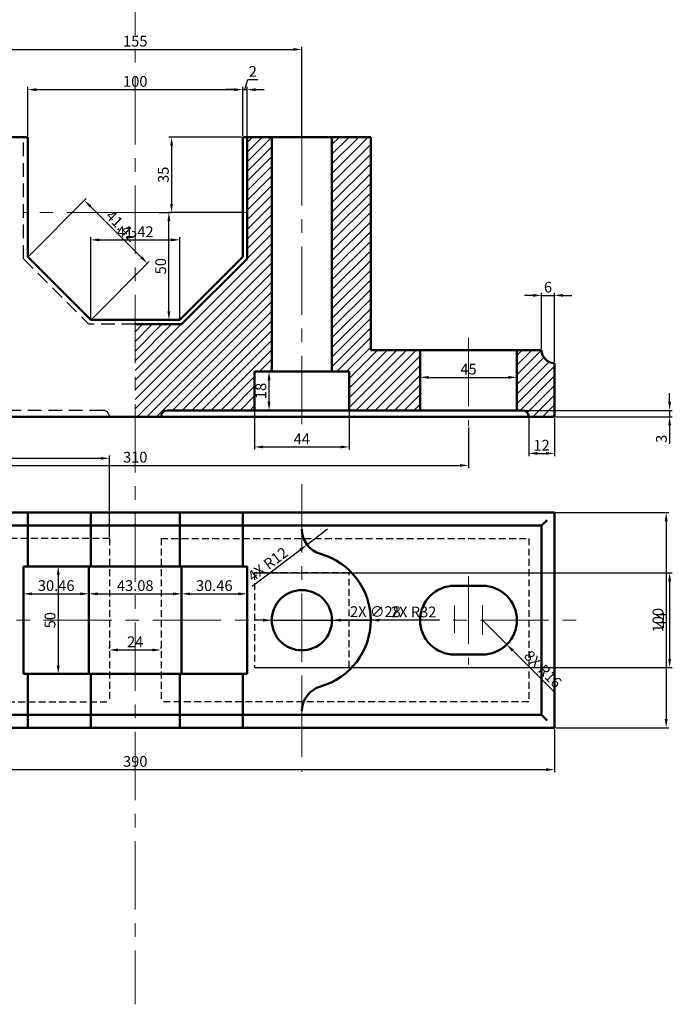
# Model space of a CAD drawing. Units: millimetres. Extents: x 3191 to 3694, y 1533 to 2269.
# Tile 2 of 2: x 3390 to 3694, y 1533 to 1990. Entities that reach past the tile are written whole.
import ezdxf

# ---------------------------------------------------------------- set-up
doc = ezdxf.new("R2010")
doc.units = ezdxf.units.MM
doc.linetypes.add('CENTER', pattern=[50.8, 31.75, -6.35, 6.35, -6.35])
doc.linetypes.add('HIDDEN', pattern=[9.525, 6.35, -3.175])
for name, color, linetype, lineweight in [('M-CNTR', 4, 'CENTER', 18), ('M-DIMS', 2, 'Continuous', 25), ('M-HATC', 8, 'Continuous', 18), ('M-HIDN', 3, 'HIDDEN', 25), ('M-OUTL', 7, 'Continuous', 50)]:
    doc.layers.add(name, color=color, linetype=linetype, lineweight=lineweight)
doc.styles.get("Standard").update_dxf_attribs({"font": 'arial.ttf'})
doc.dimstyles.new('ISO-25', dxfattribs={"dimtxt": 5, "dimasz": 4, "dimexe": 1.25, "dimexo": 0.625, "dimtad": 1, "dimdsep": 46, "dimtxsty": 'Standard', "dimcen": 2.5, "dimadec": 0, "dimazin": 0, "dimtfac": 1, "dimtmove": 0, "dimatfit": 3, "dimfxl": 1, "dimarcsym": 0})

# ---------------------------------------------------------------- blocks, each defined once
blk = doc.blocks.new('*D1')
at = {"layer": 'Defpoints', "color": 0, "ltscale": 0.5, "transparency": 16777216}
for p in [(3431.85, 1697.44), (3455.85, 1697.44), (3455.85, 1697.44)]:
    blk.add_point(p, dxfattribs=at)
at = {"layer": 'M-DIMS', "color": 0, "lineweight": -2, "ltscale": 0.5, "transparency": 16777216}
for p, q in [((3431.85, 1698.07), (3431.85, 1698.69)), ((3455.85, 1698.07), (3455.85, 1698.69)), ((3435.85, 1697.44), (3451.85, 1697.44))]:
    blk.add_line(p, q, dxfattribs=at)
at = {"layer": 'M-DIMS', "color": 0, "ltscale": 0.5, "transparency": 16777216}
for points in [[(3435.85, 1698.11), (3435.85, 1696.77), (3431.85, 1697.44)], [(3451.85, 1698.11), (3451.85, 1696.77), (3455.85, 1697.44)]]:
    blk.add_solid(points, dxfattribs=at)
at = {"layer": 'M-DIMS', "color": 0, "ltscale": 0.5, "transparency": 16777216, "insert": (3443.85, 1700.58), "char_height": 5, "attachment_point": 5}
blk.add_mtext('24', dxfattribs=at)
blk = doc.blocks.new('*D2')
at = {"layer": 'Defpoints', "color": 0, "ltscale": 0.5, "transparency": 16777216}
for p in [(3288.85, 1800.04), (3598.85, 1801.48), (3598.85, 1783.23)]:
    blk.add_point(p, dxfattribs=at)
at = {"layer": 'M-DIMS', "color": 0, "lineweight": -2, "ltscale": 0.5, "transparency": 16777216}
for p, q in [((3288.85, 1799.41), (3288.85, 1781.98)), ((3598.85, 1800.86), (3598.85, 1781.98)), ((3292.85, 1783.23), (3594.85, 1783.23))]:
    blk.add_line(p, q, dxfattribs=at)
at = {"layer": 'M-DIMS', "color": 0, "ltscale": 0.5, "transparency": 16777216}
for points in [[(3292.85, 1783.9), (3292.85, 1782.57), (3288.85, 1783.23)], [(3594.85, 1783.9), (3594.85, 1782.57), (3598.85, 1783.23)]]:
    blk.add_solid(points, dxfattribs=at)
at = {"layer": 'M-DIMS', "color": 0, "ltscale": 0.5, "transparency": 16777216, "insert": (3443.85, 1786.41), "char_height": 5, "attachment_point": 5}
blk.add_mtext('310', dxfattribs=at)
blk = doc.blocks.new('*D6')
at = {"layer": 'Defpoints', "color": 0, "ltscale": 0.5, "transparency": 16777216}
for p in [(3521.35, 1976.6), (3366.35, 1935.82), (3521.35, 1935.82)]:
    blk.add_point(p, dxfattribs=at)
at = {"layer": 'M-DIMS', "color": 0, "lineweight": -2, "ltscale": 0.5, "transparency": 16777216}
for p, q in [((3366.35, 1936.45), (3366.35, 1977.85)), ((3521.35, 1936.45), (3521.35, 1977.85)), ((3370.35, 1976.6), (3517.35, 1976.6))]:
    blk.add_line(p, q, dxfattribs=at)
at = {"layer": 'M-DIMS', "color": 0, "ltscale": 0.5, "transparency": 16777216}
for points in [[(3370.35, 1977.27), (3370.35, 1975.93), (3366.35, 1976.6)], [(3517.35, 1977.27), (3517.35, 1975.93), (3521.35, 1976.6)]]:
    blk.add_solid(points, dxfattribs=at)
at = {"layer": 'M-DIMS', "color": 0, "ltscale": 0.5, "transparency": 16777216, "insert": (3443.85, 1979.78), "char_height": 5, "attachment_point": 5}
blk.add_mtext('155', dxfattribs=at)
blk = doc.blocks.new('*D7')
at = {"layer": 'Defpoints', "color": 0, "ltscale": 0.5, "transparency": 16777216}
for p in [(3493.85, 1957.9), (3393.85, 1935.81), (3493.85, 1935.81)]:
    blk.add_point(p, dxfattribs=at)
at = {"layer": 'M-DIMS', "color": 0, "lineweight": -2, "ltscale": 0.5, "transparency": 16777216}
for p, q in [((3393.85, 1936.43), (3393.85, 1959.15)), ((3493.85, 1936.43), (3493.85, 1959.15)), ((3397.85, 1957.9), (3489.85, 1957.9))]:
    blk.add_line(p, q, dxfattribs=at)
at = {"layer": 'M-DIMS', "color": 0, "ltscale": 0.5, "transparency": 16777216}
for points in [[(3397.85, 1958.56), (3397.85, 1957.23), (3393.85, 1957.9)], [(3489.85, 1958.56), (3489.85, 1957.23), (3493.85, 1957.9)]]:
    blk.add_solid(points, dxfattribs=at)
at = {"layer": 'M-DIMS', "color": 0, "ltscale": 0.5, "transparency": 16777216, "insert": (3443.85, 1961.08), "char_height": 5, "attachment_point": 5}
blk.add_mtext('100', dxfattribs=at)
blk = doc.blocks.new('*D8')
at = {"layer": 'Defpoints', "color": 0, "ltscale": 0.5, "transparency": 16777216}
for p in [(3495.85, 1957.9), (3493.85, 1935.81), (3495.85, 1935.82)]:
    blk.add_point(p, dxfattribs=at)
at = {"layer": 'M-DIMS', "color": 0, "lineweight": -2, "ltscale": 0.5, "transparency": 16777216}
for p, q in [((3493.85, 1936.43), (3493.85, 1959.15)), ((3494.85, 1957.9), (3496.26, 1962.6)), ((3495.85, 1936.45), (3495.85, 1959.15)), ((3496.26, 1962.6), (3500.83, 1962.6)), ((3489.85, 1957.9), (3485.85, 1957.9)), ((3493.85, 1957.9), (3495.85, 1957.9)), ((3493.85, 1957.9), (3495.85, 1957.9)), ((3499.85, 1957.9), (3503.85, 1957.9))]:
    blk.add_line(p, q, dxfattribs=at)
at = {"layer": 'M-DIMS', "color": 0, "ltscale": 0.5, "transparency": 16777216}
for points in [[(3489.85, 1958.56), (3489.85, 1957.23), (3493.85, 1957.9)], [(3499.85, 1958.56), (3499.85, 1957.23), (3495.85, 1957.9)]]:
    blk.add_solid(points, dxfattribs=at)
at = {"layer": 'M-DIMS', "color": 0, "ltscale": 0.5, "transparency": 16777216, "insert": (3498.54, 1965.73), "char_height": 5, "attachment_point": 5}
blk.add_mtext('2', dxfattribs=at)
blk = doc.blocks.new('*D9')
at = {"layer": 'Defpoints', "color": 0, "ltscale": 0.5, "transparency": 16777216}
for p in [(3454.21, 1900.82), (3459.5, 1900.82), (3454.21, 1850.82)]:
    blk.add_point(p, dxfattribs=at)
at = {"layer": 'M-DIMS', "color": 0, "lineweight": -2, "ltscale": 0.5, "transparency": 16777216}
for p, q in [((3454.83, 1900.82), (3460.75, 1900.82)), ((3459.5, 1854.82), (3459.5, 1896.82)), ((3454.83, 1850.82), (3460.75, 1850.82))]:
    blk.add_line(p, q, dxfattribs=at)
at = {"layer": 'M-DIMS', "color": 0, "ltscale": 0.5, "transparency": 16777216}
for points in [[(3458.84, 1896.82), (3460.17, 1896.82), (3459.5, 1900.82)], [(3458.84, 1854.82), (3460.17, 1854.82), (3459.5, 1850.82)]]:
    blk.add_solid(points, dxfattribs=at)
at = {"layer": 'M-DIMS', "color": 0, "ltscale": 0.5, "transparency": 16777216, "insert": (3456.33, 1875.82), "char_height": 5, "attachment_point": 5, "rotation": 90}
blk.add_mtext('50', dxfattribs=at)
blk = doc.blocks.new('*D10')
at = {"layer": 'Defpoints', "color": 0, "ltscale": 0.5, "transparency": 16777216}
for p in [(3493.85, 1935.82), (3460.75, 1900.82), (3493.85, 1900.82)]:
    blk.add_point(p, dxfattribs=at)
at = {"layer": 'M-DIMS', "color": 0, "lineweight": -2, "ltscale": 0.5, "transparency": 16777216}
for p, q in [((3493.23, 1935.82), (3459.5, 1935.82)), ((3460.75, 1931.82), (3460.75, 1904.82)), ((3493.23, 1900.82), (3459.5, 1900.82))]:
    blk.add_line(p, q, dxfattribs=at)
at = {"layer": 'M-DIMS', "color": 0, "ltscale": 0.5, "transparency": 16777216}
for points in [[(3460.09, 1931.82), (3461.42, 1931.82), (3460.75, 1935.82)], [(3460.09, 1904.82), (3461.42, 1904.82), (3460.75, 1900.82)]]:
    blk.add_solid(points, dxfattribs=at)
at = {"layer": 'M-DIMS', "color": 0, "ltscale": 0.5, "transparency": 16777216, "insert": (3457.57, 1918.32), "char_height": 5, "attachment_point": 5, "rotation": 90}
blk.add_mtext('35', dxfattribs=at)
blk = doc.blocks.new('*D11')
at = {"layer": 'Defpoints', "color": 0, "ltscale": 0.5, "transparency": 16777216}
for p in [(3576.35, 1822.82), (3621.35, 1824.16), (3621.35, 1822.82)]:
    blk.add_point(p, dxfattribs=at)
at = {"layer": 'M-DIMS', "color": 0, "lineweight": -2, "ltscale": 0.5, "transparency": 16777216}
for p, q in [((3576.35, 1823.45), (3576.35, 1825.41)), ((3580.35, 1824.16), (3617.35, 1824.16)), ((3621.35, 1823.45), (3621.35, 1825.41))]:
    blk.add_line(p, q, dxfattribs=at)
at = {"layer": 'M-DIMS', "color": 0, "ltscale": 0.5, "transparency": 16777216}
for points in [[(3580.35, 1824.82), (3580.35, 1823.49), (3576.35, 1824.16)], [(3617.35, 1824.82), (3617.35, 1823.49), (3621.35, 1824.16)]]:
    blk.add_solid(points, dxfattribs=at)
at = {"layer": 'M-DIMS', "color": 0, "ltscale": 0.5, "transparency": 16777216, "insert": (3598.85, 1827.32), "char_height": 5, "attachment_point": 5}
blk.add_mtext('45', dxfattribs=at)
blk = doc.blocks.new('*D12')
at = {"layer": 'Defpoints', "color": 0, "ltscale": 0.5, "transparency": 16777216}
for p in [(3626.85, 1805.82), (3638.85, 1805.82), (3638.85, 1788.81)]:
    blk.add_point(p, dxfattribs=at)
at = {"layer": 'M-DIMS', "color": 0, "lineweight": -2, "ltscale": 0.5, "transparency": 16777216}
for p, q in [((3626.85, 1805.2), (3626.85, 1787.56)), ((3638.85, 1805.2), (3638.85, 1787.56)), ((3630.85, 1788.81), (3634.85, 1788.81))]:
    blk.add_line(p, q, dxfattribs=at)
at = {"layer": 'M-DIMS', "color": 0, "ltscale": 0.5, "transparency": 16777216}
for points in [[(3630.85, 1789.48), (3630.85, 1788.15), (3626.85, 1788.81)], [(3634.85, 1789.48), (3634.85, 1788.15), (3638.85, 1788.81)]]:
    blk.add_solid(points, dxfattribs=at)
at = {"layer": 'M-DIMS', "color": 0, "ltscale": 0.5, "transparency": 16777216, "insert": (3632.85, 1791.95), "char_height": 5, "attachment_point": 5}
blk.add_mtext('12', dxfattribs=at)
blk = doc.blocks.new('*D13')
at = {"layer": 'Defpoints', "color": 0, "ltscale": 0.5, "transparency": 16777216}
for p in [(3638.85, 1862.26), (3632.85, 1836.82), (3638.85, 1830.82)]:
    blk.add_point(p, dxfattribs=at)
at = {"layer": 'M-DIMS', "color": 0, "lineweight": -2, "ltscale": 0.5, "transparency": 16777216}
for p, q in [((3632.85, 1837.45), (3632.85, 1863.51)), ((3638.85, 1831.45), (3638.85, 1863.51)), ((3628.85, 1862.26), (3624.85, 1862.26)), ((3632.85, 1862.26), (3638.85, 1862.26)), ((3642.85, 1862.26), (3646.85, 1862.26))]:
    blk.add_line(p, q, dxfattribs=at)
at = {"layer": 'M-DIMS', "color": 0, "ltscale": 0.5, "transparency": 16777216}
for points in [[(3628.85, 1862.93), (3628.85, 1861.59), (3632.85, 1862.26)], [(3642.85, 1862.93), (3642.85, 1861.59), (3638.85, 1862.26)]]:
    blk.add_solid(points, dxfattribs=at)
at = {"layer": 'M-DIMS', "color": 0, "ltscale": 0.5, "transparency": 16777216, "insert": (3635.85, 1865.44), "char_height": 5, "attachment_point": 5}
blk.add_mtext('6', dxfattribs=at)
blk = doc.blocks.new('*D14')
at = {"layer": 'Defpoints', "color": 0, "ltscale": 0.5, "transparency": 16777216}
for p in [(3499.35, 1808.82), (3543.35, 1808.82), (3543.35, 1791.8)]:
    blk.add_point(p, dxfattribs=at)
at = {"layer": 'M-DIMS', "color": 0, "lineweight": -2, "ltscale": 0.5, "transparency": 16777216}
for p, q in [((3499.35, 1808.2), (3499.35, 1790.55)), ((3543.35, 1808.2), (3543.35, 1790.55)), ((3503.35, 1791.8), (3539.35, 1791.8))]:
    blk.add_line(p, q, dxfattribs=at)
at = {"layer": 'M-DIMS', "color": 0, "ltscale": 0.5, "transparency": 16777216}
for points in [[(3503.35, 1792.47), (3503.35, 1791.13), (3499.35, 1791.8)], [(3539.35, 1792.47), (3539.35, 1791.13), (3543.35, 1791.8)]]:
    blk.add_solid(points, dxfattribs=at)
at = {"layer": 'M-DIMS', "color": 0, "ltscale": 0.5, "transparency": 16777216, "insert": (3521.35, 1794.93), "char_height": 5, "attachment_point": 5}
blk.add_mtext('44', dxfattribs=at)
blk = doc.blocks.new('*D15')
at = {"layer": 'Defpoints', "color": 0, "ltscale": 0.5, "transparency": 16777216}
for p in [(3638.85, 1761.27), (3638.85, 1661.27), (3690.8, 1661.27)]:
    blk.add_point(p, dxfattribs=at)
at = {"layer": 'M-DIMS', "color": 0, "lineweight": -2, "ltscale": 0.5, "transparency": 16777216}
for p, q in [((3639.48, 1761.27), (3692.05, 1761.27)), ((3690.8, 1757.27), (3690.8, 1665.27)), ((3639.48, 1661.27), (3692.05, 1661.27))]:
    blk.add_line(p, q, dxfattribs=at)
at = {"layer": 'M-DIMS', "color": 0, "ltscale": 0.5, "transparency": 16777216}
for points in [[(3690.13, 1757.27), (3691.46, 1757.27), (3690.8, 1761.27)], [(3690.13, 1665.27), (3691.46, 1665.27), (3690.8, 1661.27)]]:
    blk.add_solid(points, dxfattribs=at)
at = {"layer": 'M-DIMS', "color": 0, "ltscale": 0.5, "transparency": 16777216, "insert": (3687.62, 1711.27), "char_height": 5, "attachment_point": 5, "rotation": 90}
blk.add_mtext('100', dxfattribs=at)
blk = doc.blocks.new('*D16')
at = {"layer": 'Defpoints', "color": 0, "ltscale": 0.5, "transparency": 16777216}
for p in [(3408.03, 1736.27), (3408.03, 1686.27), (3408.03, 1686.27)]:
    blk.add_point(p, dxfattribs=at)
at = {"layer": 'M-DIMS', "color": 0, "lineweight": -2, "ltscale": 0.5, "transparency": 16777216}
for p, q in [((3408.66, 1736.27), (3409.28, 1736.27)), ((3408.03, 1732.27), (3408.03, 1690.27)), ((3408.66, 1686.27), (3409.28, 1686.27))]:
    blk.add_line(p, q, dxfattribs=at)
at = {"layer": 'M-DIMS', "color": 0, "ltscale": 0.5, "transparency": 16777216}
for points in [[(3407.37, 1732.27), (3408.7, 1732.27), (3408.03, 1736.27)], [(3407.37, 1690.27), (3408.7, 1690.27), (3408.03, 1686.27)]]:
    blk.add_solid(points, dxfattribs=at)
at = {"layer": 'M-DIMS', "color": 0, "ltscale": 0.5, "transparency": 16777216, "insert": (3404.86, 1711.27), "char_height": 5, "attachment_point": 5, "rotation": 90}
blk.add_mtext('50', dxfattribs=at)
blk = doc.blocks.new('*D20')
at = {"layer": 'Defpoints', "color": 0, "ltscale": 0.5, "transparency": 16777216}
for p in [(3248.85, 1661.27), (3638.85, 1661.27), (3638.85, 1641.8)]:
    blk.add_point(p, dxfattribs=at)
at = {"layer": 'M-DIMS', "color": 0, "lineweight": -2, "ltscale": 0.5, "transparency": 16777216}
for p, q in [((3248.85, 1660.65), (3248.85, 1640.55)), ((3638.85, 1660.65), (3638.85, 1640.55)), ((3252.85, 1641.8), (3634.85, 1641.8))]:
    blk.add_line(p, q, dxfattribs=at)
at = {"layer": 'M-DIMS', "color": 0, "ltscale": 0.5, "transparency": 16777216}
for points in [[(3252.85, 1642.47), (3252.85, 1641.14), (3248.85, 1641.8)], [(3634.85, 1642.47), (3634.85, 1641.14), (3638.85, 1641.8)]]:
    blk.add_solid(points, dxfattribs=at)
at = {"layer": 'M-DIMS', "color": 0, "ltscale": 0.5, "transparency": 16777216, "insert": (3443.85, 1644.98), "char_height": 5, "attachment_point": 5}
blk.add_mtext('390', dxfattribs=at)
blk = doc.blocks.new('*D22')
at = {"layer": 'Defpoints', "color": 0, "ltscale": 0.5, "transparency": 16777216}
for p in [(3464.56, 1888.07), (3423.14, 1850.82), (3464.56, 1850.82)]:
    blk.add_point(p, dxfattribs=at)
at = {"layer": 'M-DIMS', "color": 0, "lineweight": -2, "ltscale": 0.5, "transparency": 16777216}
for p, q in [((3423.14, 1851.45), (3423.14, 1889.32)), ((3427.14, 1888.07), (3460.56, 1888.07)), ((3464.56, 1851.45), (3464.56, 1889.32))]:
    blk.add_line(p, q, dxfattribs=at)
at = {"layer": 'M-DIMS', "color": 0, "ltscale": 0.5, "transparency": 16777216}
for points in [[(3427.14, 1888.74), (3427.14, 1887.4), (3423.14, 1888.07)], [(3460.56, 1888.74), (3460.56, 1887.4), (3464.56, 1888.07)]]:
    blk.add_solid(points, dxfattribs=at)
at = {"layer": 'M-DIMS', "color": 0, "ltscale": 0.5, "transparency": 16777216, "insert": (3443.85, 1891.21), "char_height": 5, "attachment_point": 5}
blk.add_mtext('41.42', dxfattribs=at)
blk = doc.blocks.new('*D23')
at = {"layer": 'Defpoints', "color": 0, "ltscale": 0.5, "transparency": 16777216}
for p in [(3393.85, 1880.11), (3449.48, 1877.16), (3423.14, 1850.82)]:
    blk.add_point(p, dxfattribs=at)
at = {"layer": 'M-DIMS', "color": 0, "lineweight": -2, "ltscale": 0.5, "transparency": 16777216}
for p, q in [((3394.3, 1880.55), (3421.08, 1907.33)), ((3423.02, 1903.62), (3446.65, 1879.99)), ((3423.59, 1851.26), (3450.37, 1878.04))]:
    blk.add_line(p, q, dxfattribs=at)
at = {"layer": 'M-DIMS', "color": 0, "ltscale": 0.5, "transparency": 16777216}
for points in [[(3423.49, 1904.09), (3422.55, 1903.15), (3420.19, 1906.45)], [(3447.13, 1880.46), (3446.18, 1879.52), (3449.48, 1877.16)]]:
    blk.add_solid(points, dxfattribs=at)
at = {"layer": 'M-DIMS', "color": 0, "ltscale": 0.5, "transparency": 16777216, "insert": (3437.06, 1894.02), "char_height": 5, "attachment_point": 5, "rotation": 315}
blk.add_mtext('41.42', dxfattribs=at)
blk = doc.blocks.new('*D24')
at = {"layer": 'Defpoints', "color": 0, "ltscale": 0.5, "transparency": 16777216}
for p in [(3506.1, 1826.82), (3543.35, 1826.82), (3543.35, 1808.82)]:
    blk.add_point(p, dxfattribs=at)
at = {"layer": 'M-DIMS', "color": 0, "lineweight": -2, "ltscale": 0.5, "transparency": 16777216}
for p, q in [((3542.73, 1826.82), (3504.85, 1826.82)), ((3506.1, 1812.82), (3506.1, 1822.82)), ((3542.73, 1808.82), (3504.85, 1808.82))]:
    blk.add_line(p, q, dxfattribs=at)
at = {"layer": 'M-DIMS', "color": 0, "ltscale": 0.5, "transparency": 16777216}
for points in [[(3505.44, 1822.82), (3506.77, 1822.82), (3506.1, 1826.82)], [(3505.44, 1812.82), (3506.77, 1812.82), (3506.1, 1808.82)]]:
    blk.add_solid(points, dxfattribs=at)
at = {"layer": 'M-DIMS', "color": 0, "ltscale": 0.5, "transparency": 16777216, "insert": (3502.93, 1817.82), "char_height": 5, "attachment_point": 5, "rotation": 90}
blk.add_mtext('18', dxfattribs=at)
blk = doc.blocks.new('*D25')
at = {"layer": 'Defpoints', "color": 0, "ltscale": 0.5, "transparency": 16777216}
for p in [(3623.85, 1808.82), (3638.85, 1805.82), (3692.41, 1805.82)]:
    blk.add_point(p, dxfattribs=at)
at = {"layer": 'M-DIMS', "color": 0, "lineweight": -2, "ltscale": 0.5, "transparency": 16777216}
for p, q in [((3692.41, 1812.82), (3692.41, 1816.82)), ((3624.48, 1808.82), (3693.66, 1808.82)), ((3692.41, 1808.82), (3692.41, 1805.82)), ((3639.48, 1805.82), (3693.66, 1805.82)), ((3692.41, 1801.82), (3692.41, 1793.3))]:
    blk.add_line(p, q, dxfattribs=at)
at = {"layer": 'M-DIMS', "color": 0, "ltscale": 0.5, "transparency": 16777216}
for points in [[(3691.74, 1812.82), (3693.07, 1812.82), (3692.41, 1808.82)], [(3691.74, 1801.82), (3693.07, 1801.82), (3692.41, 1805.82)]]:
    blk.add_solid(points, dxfattribs=at)
at = {"layer": 'M-DIMS', "color": 0, "ltscale": 0.5, "transparency": 16777216, "insert": (3689.23, 1795.56), "char_height": 5, "attachment_point": 5, "rotation": 90}
blk.add_mtext('3', dxfattribs=at)
blk = doc.blocks.new('*D26')
at = {"layer": 'Defpoints', "color": 0, "ltscale": 0.5, "transparency": 16777216}
for p in [(3422.32, 1723.52), (3391.85, 1686.27), (3422.32, 1686.27)]:
    blk.add_point(p, dxfattribs=at)
at = {"layer": 'M-DIMS', "color": 0, "lineweight": -2, "ltscale": 0.5, "transparency": 16777216}
for p, q in [((3391.85, 1686.9), (3391.85, 1724.77)), ((3395.85, 1723.52), (3418.32, 1723.52)), ((3422.32, 1686.9), (3422.32, 1724.77))]:
    blk.add_line(p, q, dxfattribs=at)
at = {"layer": 'M-DIMS', "color": 0, "ltscale": 0.5, "transparency": 16777216}
for points in [[(3395.85, 1724.19), (3395.85, 1722.86), (3391.85, 1723.52)], [(3418.32, 1724.19), (3418.32, 1722.86), (3422.32, 1723.52)]]:
    blk.add_solid(points, dxfattribs=at)
at = {"layer": 'M-DIMS', "color": 0, "ltscale": 0.5, "transparency": 16777216, "insert": (3407.08, 1726.7), "char_height": 5, "attachment_point": 5}
blk.add_mtext('30.46', dxfattribs=at)
blk = doc.blocks.new('*D27')
at = {"layer": 'Defpoints', "color": 0, "ltscale": 0.5, "transparency": 16777216}
for p in [(3465.39, 1723.52), (3422.32, 1686.27), (3465.39, 1686.27)]:
    blk.add_point(p, dxfattribs=at)
at = {"layer": 'M-DIMS', "color": 0, "lineweight": -2, "ltscale": 0.5, "transparency": 16777216}
for p, q in [((3422.32, 1686.9), (3422.32, 1724.77)), ((3426.32, 1723.52), (3461.39, 1723.52)), ((3465.39, 1686.9), (3465.39, 1724.77))]:
    blk.add_line(p, q, dxfattribs=at)
at = {"layer": 'M-DIMS', "color": 0, "ltscale": 0.5, "transparency": 16777216}
for points in [[(3426.32, 1724.19), (3426.32, 1722.86), (3422.32, 1723.52)], [(3461.39, 1724.19), (3461.39, 1722.86), (3465.39, 1723.52)]]:
    blk.add_solid(points, dxfattribs=at)
at = {"layer": 'M-DIMS', "color": 0, "ltscale": 0.5, "transparency": 16777216, "insert": (3443.85, 1726.7), "char_height": 5, "attachment_point": 5}
blk.add_mtext('43.08', dxfattribs=at)
blk = doc.blocks.new('*D28')
at = {"layer": 'Defpoints', "color": 0, "ltscale": 0.5, "transparency": 16777216}
for p in [(3495.85, 1723.52), (3465.39, 1686.27), (3495.85, 1686.27)]:
    blk.add_point(p, dxfattribs=at)
at = {"layer": 'M-DIMS', "color": 0, "lineweight": -2, "ltscale": 0.5, "transparency": 16777216}
for p, q in [((3465.39, 1686.9), (3465.39, 1724.77)), ((3469.39, 1723.52), (3491.85, 1723.52)), ((3495.85, 1686.9), (3495.85, 1724.77))]:
    blk.add_line(p, q, dxfattribs=at)
at = {"layer": 'M-DIMS', "color": 0, "ltscale": 0.5, "transparency": 16777216}
for points in [[(3469.39, 1724.19), (3469.39, 1722.86), (3465.39, 1723.52)], [(3491.85, 1724.19), (3491.85, 1722.86), (3495.85, 1723.52)]]:
    blk.add_solid(points, dxfattribs=at)
at = {"layer": 'M-DIMS', "color": 0, "ltscale": 0.5, "transparency": 16777216, "insert": (3480.62, 1726.7), "char_height": 5, "attachment_point": 5}
blk.add_mtext('30.46', dxfattribs=at)
blk = doc.blocks.new('*D29')
at = {"layer": 'Defpoints', "color": 0, "ltscale": 0.5, "transparency": 16777216}
for p in [(3431.85, 1786.52), (3260.85, 1749.27), (3431.85, 1749.27)]:
    blk.add_point(p, dxfattribs=at)
at = {"layer": 'M-DIMS', "color": 0, "lineweight": -2, "ltscale": 0.5, "transparency": 16777216}
for p, q in [((3260.85, 1749.9), (3260.85, 1787.77)), ((3264.85, 1786.52), (3427.85, 1786.52)), ((3431.85, 1749.9), (3431.85, 1787.77))]:
    blk.add_line(p, q, dxfattribs=at)
at = {"layer": 'M-DIMS', "color": 0, "ltscale": 0.5, "transparency": 16777216}
for points in [[(3264.85, 1787.19), (3264.85, 1785.86), (3260.85, 1786.52)], [(3427.85, 1787.19), (3427.85, 1785.86), (3431.85, 1786.52)]]:
    blk.add_solid(points, dxfattribs=at)
at = {"layer": 'M-DIMS', "color": 0, "ltscale": 0.5, "transparency": 16777216, "insert": (3346.35, 1789.66), "char_height": 5, "attachment_point": 5}
blk.add_mtext('171', dxfattribs=at)
blk = doc.blocks.new('*D32')
at = {"layer": 'Defpoints', "color": 0, "ltscale": 0.5, "transparency": 16777216}
for p in [(3499.35, 1733.27), (3499.35, 1689.27), (3692.41, 1689.27)]:
    blk.add_point(p, dxfattribs=at)
at = {"layer": 'M-DIMS', "color": 0, "lineweight": -2, "ltscale": 0.5, "transparency": 16777216}
for p, q in [((3499.98, 1733.27), (3693.66, 1733.27)), ((3692.41, 1729.27), (3692.41, 1693.27)), ((3499.98, 1689.27), (3693.66, 1689.27))]:
    blk.add_line(p, q, dxfattribs=at)
at = {"layer": 'M-DIMS', "color": 0, "ltscale": 0.5, "transparency": 16777216}
for points in [[(3691.74, 1729.27), (3693.07, 1729.27), (3692.41, 1733.27)], [(3691.74, 1693.27), (3693.07, 1693.27), (3692.41, 1689.27)]]:
    blk.add_solid(points, dxfattribs=at)
at = {"layer": 'M-DIMS', "color": 0, "ltscale": 0.5, "transparency": 16777216, "insert": (3689.28, 1711.27), "char_height": 5, "attachment_point": 5, "rotation": 90}
blk.add_mtext('44', dxfattribs=at)
blk = doc.blocks.new('*D33')
at = {"layer": 'Defpoints', "color": 0, "ltscale": 0.5, "transparency": 16777216}
for p in [(3533.35, 1753.6), (3523.78, 1746.37)]:
    blk.add_point(p, dxfattribs=at)
at = {"layer": 'M-DIMS', "color": 0, "lineweight": -2, "ltscale": 0.5, "transparency": 16777216}
for p, q in [((3533.35, 1753.6), (3523.78, 1746.37)), ((3498.18, 1727.02), (3520.59, 1743.96))]:
    blk.add_line(p, q, dxfattribs=at)
at = {"layer": 'M-DIMS', "color": 0, "ltscale": 0.5, "transparency": 16777216}
blk.add_solid([(3520.19, 1744.49), (3520.99, 1743.42), (3523.78, 1746.37)], dxfattribs=at)
at = {"layer": 'M-DIMS', "color": 0, "ltscale": 0.5, "transparency": 16777216, "insert": (3505.9, 1736.78), "char_height": 5, "attachment_point": 5, "rotation": 37.0868}
blk.add_mtext('4X R12', dxfattribs=at)
blk = doc.blocks.new('*D34')
at = {"layer": 'Defpoints', "color": 0, "ltscale": 0.5, "transparency": 16777216}
for p in [(3521.35, 1711.27), (3553.35, 1711.27)]:
    blk.add_point(p, dxfattribs=at)
at = {"layer": 'M-DIMS', "color": 0, "lineweight": -2, "ltscale": 0.5, "transparency": 16777216}
for p, q in [((3521.35, 1711.27), (3553.35, 1711.27)), ((3585.33, 1711.27), (3557.35, 1711.27))]:
    blk.add_line(p, q, dxfattribs=at)
at = {"layer": 'M-DIMS', "color": 0, "ltscale": 0.5, "transparency": 16777216}
blk.add_solid([(3557.35, 1711.94), (3557.35, 1710.61), (3553.35, 1711.27)], dxfattribs=at)
at = {"layer": 'M-DIMS', "color": 0, "ltscale": 0.5, "transparency": 16777216, "insert": (3573.34, 1714.45), "char_height": 5, "attachment_point": 5, "rotation": 0.0006}
blk.add_mtext('2X R32', dxfattribs=at)
blk = doc.blocks.new('*D35')
at = {"layer": 'Defpoints', "color": 0, "ltscale": 0.5, "transparency": 16777216}
for p in [(3605.35, 1711.27), (3616.67, 1699.96)]:
    blk.add_point(p, dxfattribs=at)
at = {"layer": 'M-DIMS', "color": 0, "lineweight": -2, "ltscale": 0.5, "transparency": 16777216}
for p, q in [((3605.35, 1711.27), (3616.67, 1699.96)), ((3639.26, 1677.37), (3619.5, 1697.13))]:
    blk.add_line(p, q, dxfattribs=at)
at = {"layer": 'M-DIMS', "color": 0, "ltscale": 0.5, "transparency": 16777216}
blk.add_solid([(3619.97, 1697.6), (3619.03, 1696.66), (3616.67, 1699.96)], dxfattribs=at)
at = {"layer": 'M-DIMS', "color": 0, "ltscale": 0.5, "transparency": 16777216, "insert": (3633.04, 1688.08), "char_height": 5, "attachment_point": 5, "rotation": 315.0005}
blk.add_mtext('8X R16', dxfattribs=at)
blk = doc.blocks.new('*D36')
at = {"layer": 'Defpoints', "color": 0, "ltscale": 0.5, "transparency": 16777216}
for p in [(3507.35, 1711.27), (3535.35, 1711.27)]:
    blk.add_point(p, dxfattribs=at)
at = {"layer": 'M-DIMS', "color": 0, "lineweight": -2, "ltscale": 0.5, "transparency": 16777216}
for p, q in [((3503.35, 1711.27), (3499.35, 1711.27)), ((3507.35, 1711.27), (3535.35, 1711.27)), ((3567.78, 1711.27), (3539.35, 1711.27))]:
    blk.add_line(p, q, dxfattribs=at)
at = {"layer": 'M-DIMS', "color": 0, "ltscale": 0.5, "transparency": 16777216}
for points in [[(3503.35, 1711.94), (3503.35, 1710.61), (3507.35, 1711.27)], [(3539.35, 1711.94), (3539.35, 1710.61), (3535.35, 1711.27)]]:
    blk.add_solid(points, dxfattribs=at)
at = {"layer": 'M-DIMS', "color": 0, "ltscale": 0.5, "transparency": 16777216, "insert": (3555.57, 1714.59), "char_height": 5, "attachment_point": 5, "rotation": 0.0015}
blk.add_mtext('2X ∅28', dxfattribs=at)

msp = doc.modelspace()

# ---------------------------------------------------------------- hatches: boundary and pattern name
at = {"layer": 'M-HATC', "ltscale": 0.5}
h = msp.add_hatch(dxfattribs=at)
h.set_pattern_fill('ANSI31', color=256)
h.paths.add_polyline_path([(3507.354, 1935.82), (3495.854, 1935.82), (3495.854, 1879.281), (3465.393, 1848.82), (3443.854, 1848.82), (3443.854, 1805.82), (3455.854, 1805.82, -0.4142136), (3458.854, 1808.82), (3499.354, 1808.82), (3499.354, 1826.82), (3507.354, 1826.82)])
h.paths.add_polyline_path([(3553.354, 1935.82), (3535.354, 1935.82), (3535.354, 1826.82), (3543.354, 1826.82), (3543.354, 1808.82), (3576.354, 1808.82), (3576.354, 1836.82), (3553.354, 1836.82)])
h.paths.add_polyline_path([(3638.854, 1830.82, -0.4142136), (3632.854, 1836.82), (3621.354, 1836.82), (3621.354, 1808.82), (3623.854, 1808.82, -0.4142136), (3626.854, 1805.82), (3638.854, 1805.82)])

# ---------------------------------------------------------------- linework, layer by layer
at = {"layer": 'M-CNTR'}
for p, q in [((3443.854, 2268.929), (3443.854, 1532.711)), ((3521.354, 1935.82), (3521.354, 1798.916)), ((3443.854, 1900.82), (3391.854, 1900.82)), ((3443.854, 1900.82), (3495.854, 1900.82)), ((3598.854, 1842.565), (3598.854, 1801.484)), ((3521.354, 1774.44), (3521.354, 1679.273)), ((3598.854, 1731.813), (3598.854, 1690.732)), ((3592.354, 1718.09), (3592.354, 1705.282)), ((3605.354, 1718.256), (3605.354, 1704.494)), ((3248.854, 1711.273), (3655.157, 1711.273)), ((3521.354, 1679.273), (3521.354, 1640.763))]:
    msp.add_line(p, q, dxfattribs=at)
at = {"layer": 'M-HIDN'}
for p, q in [((3391.854, 1879.281), (3391.854, 1935.82)), ((3391.854, 1879.281), (3422.315, 1848.82)), ((3443.854, 1848.82), (3422.315, 1848.82)), ((3428.854, 1808.82), (3263.854, 1808.82))]:
    msp.add_line(p, q, dxfattribs=at)
at = {"layer": 'M-HIDN', "ltscale": 0.5}
for p, q in [((3431.854, 1749.273), (3260.854, 1749.273)), ((3431.854, 1749.273), (3431.854, 1673.273)), ((3455.854, 1749.273), (3626.854, 1749.273)), ((3455.854, 1749.273), (3455.854, 1673.273)), ((3626.854, 1749.273), (3626.854, 1673.273)), ((3260.854, 1673.273), (3431.854, 1673.273)), ((3626.854, 1673.273), (3455.854, 1673.273))]:
    msp.add_line(p, q, dxfattribs=at)
msp.add_lwpolyline([(3543.354, 1733.273), (3499.354, 1733.273), (3499.354, 1689.273), (3543.354, 1689.273)], close=True, dxfattribs=at)
at = {"layer": 'M-HIDN'}
msp.add_arc((3428.854, 1805.82), 3, 0, 90, dxfattribs=at)
at = {"layer": 'M-OUTL'}
for p, q in [((3393.854, 1935.82), (3334.354, 1935.82)), ((3393.854, 1880.109), (3393.854, 1935.82)), ((3493.854, 1880.109), (3493.854, 1935.82)), ((3493.854, 1935.82), (3553.354, 1935.82)), ((3495.854, 1879.281), (3495.854, 1935.82)), ((3507.354, 1935.82), (3507.354, 1826.82)), ((3535.354, 1935.82), (3535.354, 1826.82)), ((3553.354, 1935.82), (3553.354, 1836.82)), ((3423.143, 1850.82), (3393.854, 1880.109)), ((3464.565, 1850.82), (3493.854, 1880.109)), ((3465.393, 1848.82), (3495.854, 1879.281)), ((3443.854, 1850.82), (3423.143, 1850.82)), ((3443.854, 1850.82), (3464.565, 1850.82)), ((3443.854, 1848.82), (3465.393, 1848.82)), ((3553.354, 1836.82), (3632.854, 1836.82)), ((3576.354, 1836.82), (3576.354, 1808.82)), ((3621.354, 1836.82), (3621.354, 1808.82)), ((3499.354, 1826.82), (3499.354, 1808.82)), ((3499.354, 1826.82), (3543.354, 1826.82)), ((3543.354, 1826.82), (3543.354, 1808.82)), ((3638.854, 1830.82), (3638.854, 1805.82)), ((3458.854, 1808.82), (3623.854, 1808.82)), ((3443.854, 1805.82), (3248.854, 1805.82)), ((3443.854, 1805.82), (3638.854, 1805.82))]:
    msp.add_line(p, q, dxfattribs=at)
at = {"layer": 'M-OUTL', "ltscale": 0.5}
for p, q in [((3443.854, 1761.273), (3248.854, 1761.273)), ((3393.854, 1761.273), (3393.854, 1736.273)), ((3423.143, 1761.273), (3423.143, 1736.273)), ((3443.854, 1761.273), (3638.854, 1761.273)), ((3464.565, 1761.273), (3464.565, 1736.273)), ((3493.854, 1761.273), (3493.854, 1736.273)), ((3632.854, 1755.273), (3635.412, 1757.83)), ((3638.854, 1761.273), (3638.854, 1661.273)), ((3443.854, 1755.273), (3254.854, 1755.273)), ((3443.854, 1755.273), (3632.854, 1755.273)), ((3632.854, 1755.273), (3632.854, 1667.273)), ((3443.854, 1736.273), (3391.854, 1736.273)), ((3391.854, 1736.273), (3391.854, 1711.273)), ((3422.315, 1736.273), (3422.315, 1711.273)), ((3443.854, 1736.273), (3495.854, 1736.273)), ((3465.393, 1736.273), (3465.393, 1711.273)), ((3495.854, 1736.273), (3495.854, 1711.273)), ((3391.854, 1686.273), (3391.854, 1711.273)), ((3422.315, 1686.273), (3422.315, 1711.273)), ((3465.393, 1686.273), (3465.393, 1711.273)), ((3495.854, 1686.273), (3495.854, 1711.273)), ((3443.854, 1686.273), (3391.854, 1686.273)), ((3393.854, 1661.273), (3393.854, 1686.273)), ((3423.143, 1661.273), (3423.143, 1686.273)), ((3443.854, 1686.273), (3495.854, 1686.273)), ((3464.565, 1661.273), (3464.565, 1686.273)), ((3493.854, 1661.273), (3493.854, 1686.273)), ((3254.854, 1667.273), (3443.854, 1667.273)), ((3632.854, 1667.273), (3443.854, 1667.273)), ((3632.854, 1667.273), (3635.412, 1664.715)), ((3248.854, 1661.273), (3443.854, 1661.273)), ((3638.854, 1661.273), (3443.854, 1661.273))]:
    msp.add_line(p, q, dxfattribs=at)
msp.add_lwpolyline([(3621.354, 1711.273, -0.4142136), (3605.354, 1695.273), (3592.354, 1695.273, -0.4142136), (3576.354, 1711.273), (3576.354, 1711.273, -0.4142136), (3592.354, 1727.273), (3605.354, 1727.273, -0.4142136), (3621.354, 1711.273)], format="xyb", close=True, dxfattribs=at)
msp.add_circle((3521.354, 1711.273), 14, dxfattribs=at)
at = {"layer": 'M-OUTL'}
for centre, radius, start, end in [((3638.854, 1836.82), 6, 180, 270), ((3458.854, 1805.82), 3, 90, 180), ((3623.854, 1805.82), 3, 0, 90)]:
    msp.add_arc(centre, radius, start, end, dxfattribs=at)
at = {"layer": 'M-OUTL', "ltscale": 0.5}
for centre, radius, start, end in [((3533.354, 1753.605), 12, 180, 254.17338), ((3521.354, 1711.273), 32, 285.82662, 74.17338), ((3533.354, 1668.941), 12, 105.82662, 180)]:
    msp.add_arc(centre, radius, start, end, dxfattribs=at)

# ---------------------------------------------------------------- dimensions: what is measured, and where the dimension line sits
at = {"layer": 'M-DIMS', "ltscale": 0.5}
for base, p1, p2, override, picture, middle in [((3521.354, 1976.6), (3366.354, 1935.82), (3521.354, 1935.82), {"dimclrd": 0, "dimclre": 0, "dimclrt": 0}, '*D6', (3443.854, 1979.777)), ((3495.854, 1957.898), (3493.854, 1935.809), (3495.854, 1935.82), {"dimclrd": 0, "dimclre": 0, "dimclrt": 0, "dimtmove": 1}, '*D8', (3496.888, 1965.731)), ((3493.854, 1957.898), (3393.854, 1935.809), (3493.854, 1935.809), {"dimclrd": 0, "dimclre": 0, "dimclrt": 0}, '*D7', (3443.854, 1961.076)), ((3464.565, 1888.07), (3423.143, 1850.82), (3464.565, 1850.82), {"dimdec": 2, "dimlfac": 1, "dimrnd": 0, "dimzin": 0, "dimdsep": 46, "dimlunit": 2}, '*D22', (3443.854, 1891.205)), ((3638.854, 1862.259), (3632.854, 1836.82), (3638.854, 1830.82), {"dimclrd": 0, "dimclre": 0, "dimclrt": 0}, '*D13', (3635.854, 1865.437)), ((3621.354, 1824.155), (3576.354, 1822.82), (3621.354, 1822.82), {"dimclrd": 0, "dimclre": 0, "dimclrt": 0}, '*D11', (3598.854, 1827.323)), ((3543.354, 1791.801), (3499.354, 1808.82), (3543.354, 1808.82), {"dimclrd": 0, "dimclre": 0, "dimclrt": 0}, '*D14', (3521.354, 1794.926)), ((3638.854, 1788.813), (3626.854, 1805.82), (3638.854, 1805.82), {"dimclrd": 0, "dimclre": 0, "dimclrt": 0}, '*D12', (3632.854, 1791.948)), ((3598.854, 1783.232), (3288.854, 1800.036), (3598.854, 1801.484), {"dimclrd": 0, "dimclre": 0, "dimclrt": 0}, '*D2', (3443.854, 1786.412)), ((3431.854, 1786.523), (3260.854, 1749.273), (3431.854, 1749.273), {"dimdec": 0, "dimlfac": 1, "dimrnd": 0, "dimzin": 0, "dimdsep": 46, "dimlunit": 2}, '*D29', (3346.354, 1789.658)), ((3422.315, 1723.523), (3391.854, 1686.273), (3422.315, 1686.273), {"dimdec": 2, "dimlfac": 1, "dimrnd": 0, "dimzin": 0, "dimdsep": 46, "dimlunit": 2}, '*D26', (3407.085, 1726.702)), ((3465.393, 1723.523), (3422.315, 1686.273), (3465.393, 1686.273), {"dimdec": 2, "dimlfac": 1, "dimrnd": 0, "dimzin": 0, "dimdsep": 46, "dimlunit": 2}, '*D27', (3443.854, 1726.702)), ((3495.854, 1723.523), (3465.393, 1686.273), (3495.854, 1686.273), {"dimdec": 2, "dimlfac": 1, "dimrnd": 0, "dimzin": 0, "dimdsep": 46, "dimlunit": 2}, '*D28', (3480.624, 1726.702)), ((3455.854, 1697.442), (3431.854, 1697.442), (3455.854, 1697.442), {"dimclrd": 0, "dimclre": 0, "dimclrt": 0}, '*D1', (3443.854, 1700.577)), ((3638.854, 1641.804), (3248.854, 1661.273), (3638.854, 1661.273), {"dimclrd": 0, "dimclre": 0, "dimclrt": 0}, '*D20', (3443.854, 1644.984))]:
    dim = msp.add_linear_dim(base=base, p1=p1, p2=p2, dimstyle='ISO-25', override=override, dxfattribs=at)
    dim.commit()
    dim.dimension.update_dxf_attribs({"geometry": picture, "text_midpoint": middle})
for base, p1, p2, angle, override, picture, middle in [((3460.753, 1900.82), (3493.854, 1935.82), (3493.854, 1900.82), 90, {"dimclrd": 0, "dimclre": 0, "dimclrt": 0}, '*D10', (3457.573, 1918.32)), ((3449.483, 1877.16), (3393.854, 1880.109), (3423.143, 1850.82), 315, {"dimdec": 2, "dimlfac": 1, "dimrnd": 0, "dimzin": 0, "dimdsep": 46, "dimlunit": 2}, '*D23', (3437.055, 1894.021)), ((3459.503, 1900.82), (3454.209, 1850.82), (3454.209, 1900.82), 90, {"dimclrd": 0, "dimclre": 0, "dimclrt": 0}, '*D9', (3456.325, 1875.82)), ((3506.104, 1826.82), (3543.354, 1808.82), (3543.354, 1826.82), 90, {"dimdec": 0, "dimlfac": 1, "dimrnd": 0, "dimzin": 0, "dimdsep": 46, "dimlunit": 2}, '*D24', (3502.926, 1817.82)), ((3692.407, 1805.82), (3623.854, 1808.82), (3638.854, 1805.82), 90, {"dimdec": 0, "dimlfac": 1, "dimrnd": 0, "dimzin": 0, "dimdsep": 46, "dimlunit": 2}, '*D25', (3689.227, 1795.558)), ((3690.797, 1661.273), (3638.854, 1761.273), (3638.854, 1661.273), 90, {"dimclrd": 0, "dimclre": 0, "dimclrt": 0}, '*D15', (3687.619, 1711.273)), ((3692.407, 1689.273), (3499.354, 1733.273), (3499.354, 1689.273), 90, {"dimdec": 0, "dimlfac": 1, "dimrnd": 0, "dimzin": 0, "dimdsep": 46, "dimlunit": 2}, '*D32', (3689.282, 1711.273))]:
    dim = msp.add_linear_dim(base=base, p1=p1, p2=p2, angle=angle, dimstyle='ISO-25', override=override, dxfattribs=at)
    dim.commit()
    dim.dimension.update_dxf_attribs({"geometry": picture, "text_midpoint": middle})
for center, mpoint, text, picture, middle in [((3533.354, 1753.605), (3523.781, 1746.368), '4X <>', '*D33', (3505.899, 1736.783)), ((3521.354, 1711.273), (3553.354, 1711.273), '2X <>', '*D34', (3573.342, 1714.453)), ((3605.354, 1711.273), (3616.668, 1699.959), '8X <>', '*D35', (3633.038, 1688.084))]:
    dim = msp.add_radius_dim(center=center, mpoint=mpoint, text=text, dimstyle='ISO-25', override={"dimdec": 0, "dimlfac": 1, "dimrnd": 0, "dimzin": 0, "dimdsep": 46, "dimlunit": 2}, dxfattribs=at)
    dim.commit()
    dim.dimension.update_dxf_attribs({"geometry": picture, "text_midpoint": middle})
dim = msp.add_aligned_dim(p1=(3408.033, 1736.273), p2=(3408.033, 1686.273), distance=0, dimstyle='ISO-25', override={"dimclrd": 0, "dimclre": 0, "dimclrt": 0}, dxfattribs=at)
dim.commit()
dim.dimension.update_dxf_attribs({"geometry": '*D16', "text_midpoint": (3404.855, 1711.273)})
dim = msp.add_diameter_dim_2p(p1=(3507.354, 1711.272), p2=(3535.354, 1711.273), text='2X <>', dimstyle='ISO-25', override={"dimdec": 0, "dimlfac": 1, "dimrnd": 0, "dimzin": 0, "dimdsep": 46, "dimlunit": 2}, dxfattribs=at)
dim.commit()
dim.dimension.update_dxf_attribs({"geometry": '*D36', "text_midpoint": (3555.567, 1711.274), "dimtype": 163})

doc.saveas('drawing.dxf')
